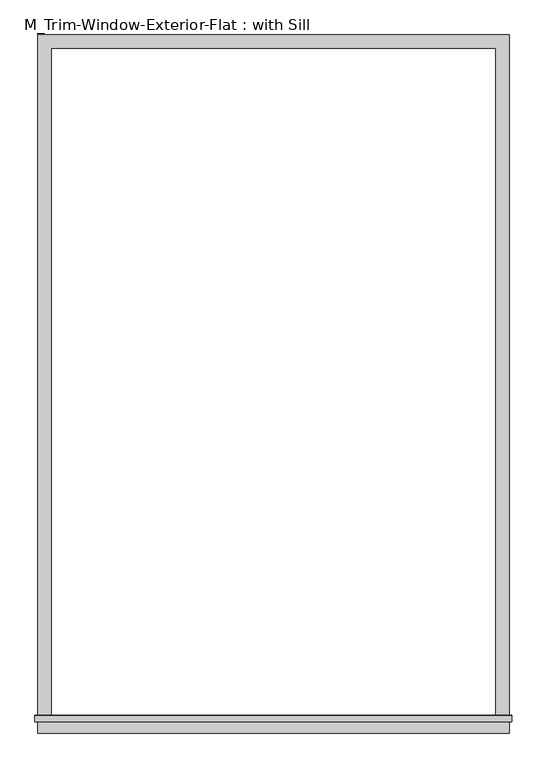
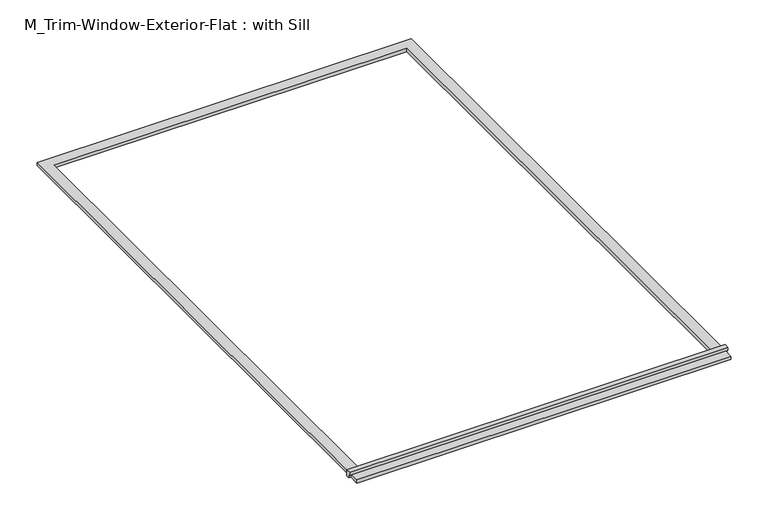
"""IFC4 building model written with IfcOpenShell, lengths in millimetres: proxy geometry, M_Trim-Window-Exterior-Flat : with Sill."""

from ifc_helpers import new_model, si_unit, frame, origin, origin_with_axes, place, context, project, spatial, polyline, outline, extrude, source, transform, mapped, element, save


def m_trim_window_exterior_flat_with_sill_5e8edc4f(model_context):
    return source(origin(), model_context, "Body", "SweptSolid", [
        extrude(outline(polyline([(1060.0, -3020.4323709), (1060.0, -3080.4323709), (-1060.0, -3080.4323709), (-1060.0, -3020.4323709), (1060.0, -3020.4323709)])), origin_with_axes(), (0.0, 0.0, 1.0), 19.05),
        extrude(outline(polyline([(-3030.0, 38.1), (-3002.4580645, 38.1), (-3000.0, 19.05), (-3000.0, 0.0), (-3020.4323709, 0.0), (-3020.4323709, 19.05), (-3030.0, 19.05), (-3030.0, 38.1)])), frame((-1072.7, 0.0, 0.0), z_axis=(1.0, 0.0, 0.0), x_axis=(0.0, 1.0, 0.0)), (0.0, 0.0, 1.0), 2145.4),
        extrude(outline(polyline([(-1060.0, 60.0), (1060.0, 60.0), (1060.0, -3000.0), (1000.0, -3000.0), (1000.0, 0.0), (-1000.0, 0.0), (-1000.0, -3000.0), (-1060.0, -3000.0), (-1060.0, 60.0)])), origin_with_axes(), (0.0, 0.0, 1.0), 19.05),
    ])


if __name__ == "__main__":
    model = new_model("IFC4")
    model_context = context("Model", 3, world=origin())
    ifc_project = project(units=[si_unit("LENGTHUNIT", "METRE", prefix="MILLI")], contexts=[model_context])
    site = spatial("IfcSite", under=ifc_project)
    building = spatial("IfcBuilding", under=site)
    placement = place(None, origin())
    m_trim_window_exterior_flat_with_sill_shape = m_trim_window_exterior_flat_with_sill_5e8edc4f(model_context)
    element("IfcBuildingElementProxy", 1, Name="M_Trim-Window-Exterior-Flat : with Sill", ObjectType="M_Trim-Window-Exterior-Flat : with Sill", at=placement, inside=building, context=model_context, shape_type="MappedRepresentation", body=[
        mapped(m_trim_window_exterior_flat_with_sill_shape, transform((0.0, 0.0, 0.0), x_axis=(1.0, 0.0, 0.0), y_axis=(0.0, 1.0, 0.0), z_axis=(0.0, 0.0, 1.0))),
    ])
    save(model, "model.ifc")

# Revit data of these elements
# Type "M_Trim-Window-Exterior-Flat : with Sill"
#   Trim Width = 60 mm
#   Trim Thickness_Picture Frame = 30 mm
#   Trim Thickness_with Sill = 19.05 mm
#   Sill Thickness = 30 mm
#   Opening Width [instance default] = 600 mm
#   Opening Height [instance default] = 900 mm
#   Default Elevation = 1200 mm
#   Sill = yes
#   Picture Frame = no
#   Trim Material [instance default] = none
# Element 1 (IfcBuildingElementProxy, "M_Trim-Window-Exterior-Flat : with Sill")
#   Opening Width = 2000 mm
#   Opening Height = 3000 mm
#   Trim Material = Clad - White
#   Materials on its faces: "Clad - White"
# Materials
#   "Clad - White": class "Wood", colour RGB 242 242 238, transparency 0, Cost = 0
